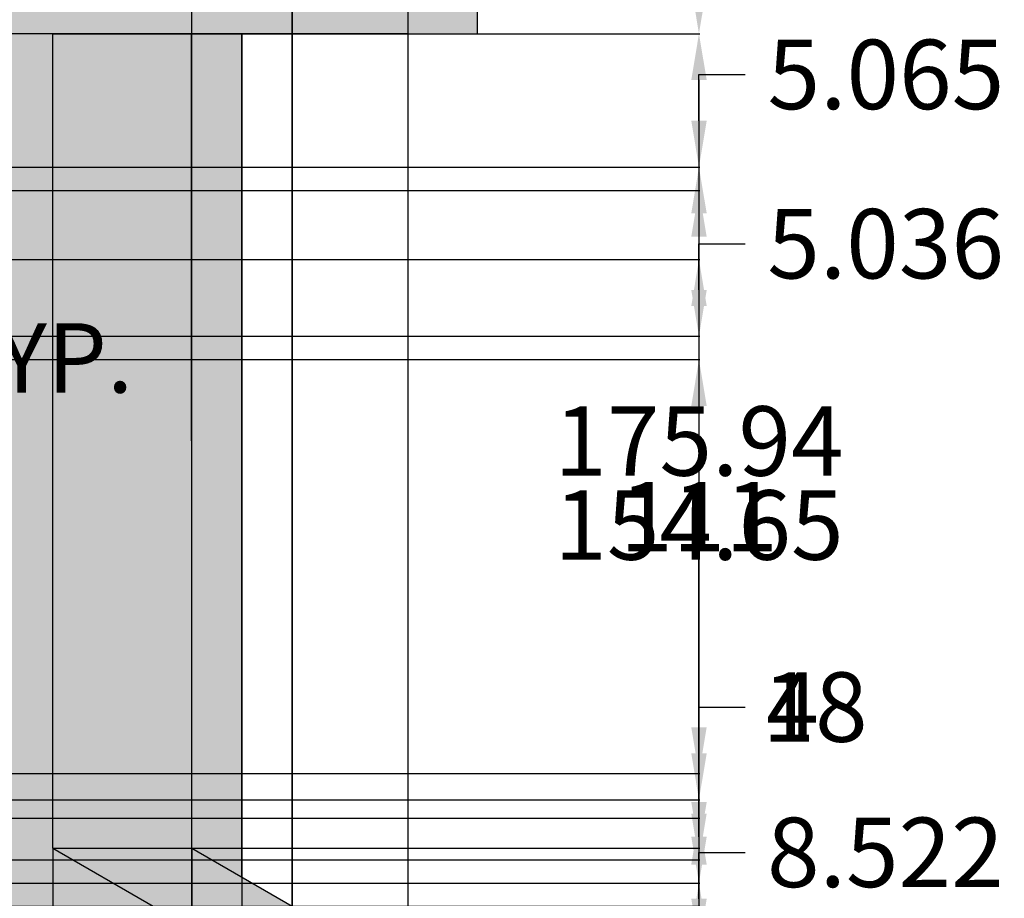
# Model space of a CAD drawing. Units: millimetres. Extents: x 131 to 845, y -20 to 1043.
# Tile 8 of 11: x 622 to 834, y 302 to 492. Entities that reach past the tile are written whole.
import ezdxf

# ---------------------------------------------------------------- set-up
doc = ezdxf.new("R2010")
doc.units = ezdxf.units.MM
doc.header["$MEASUREMENT"] = 0
for name, color, linetype, lineweight in [('A-ANNO-DIMS', 2, 'Continuous', 18), ('A-ELEV', 7, 'Continuous', 25), ('A-ELEV-PATT', 7, 'Continuous', 13), ('A-GLAZ-PATT', 143, 'Continuous', 13), ('A-WALL-PATT', 131, 'Continuous', 13)]:
    doc.layers.add(name, color=color, linetype=linetype, lineweight=lineweight)
doc.styles.get("Standard").update_dxf_attribs({"font": 'arial.ttf'})
doc.dimstyles.get("Standard").update_dxf_attribs({"dimtxt": 15, "dimasz": 10, "dimexe": 0.18, "dimexo": 0.0625, "dimgap": 5, "dimtad": 0, "dimtih": 1, "dimtoh": 1, "dimdec": 0, "dimzin": 0, "dimdsep": 46, "dimtxsty": 'Standard', "dimcen": 5, "dimadec": 0, "dimazin": 0, "dimtfac": 1, "dimtdec": 0, "dimtofl": 0, "dimtmove": 0, "dimatfit": 3, "dimfxl": 1, "dimtolj": 1, "dimtzin": 0, "dimarcsym": 0})

# ---------------------------------------------------------------- blocks, each defined once
blk = doc.blocks.new('*D12')
at = {"layer": 'A-ANNO-DIMS', "color": 0, "lineweight": -2, "transparency": 16777216}
for p, q in [((530.07, 423.18), (530.08, 418.34)), ((550.07, 423.21), (550.08, 418.36)), ((520.08, 418.5), (510.08, 418.49)), ((560.08, 418.56), (570.08, 418.57))]:
    blk.add_line(p, q, dxfattribs=at)
at = {"layer": 'A-ANNO-DIMS', "color": 0, "transparency": 16777216}
for points in [[(520.07, 420.17), (520.08, 416.83), (530.08, 418.52)], [(560.07, 420.22), (560.08, 416.89), (550.08, 418.54)]]:
    blk.add_solid(points, dxfattribs=at)
at = {"layer": 'Defpoints', "color": 0, "transparency": 16777216}
for p in [(530.07, 423.24), (550.07, 423.27), (550.08, 418.54)]:
    blk.add_point(p, dxfattribs=at)
at = {"layer": 'A-ANNO-DIMS', "color": 0, "transparency": 16777216, "insert": (611.71, 418.57), "char_height": 15, "attachment_point": 5}
blk.add_mtext('\\A1;20 TYP.', dxfattribs=at)
blk = doc.blocks.new('*D40')
at = {"layer": 'A-ANNO-DIMS', "color": 0, "lineweight": -2, "transparency": 16777216}
for p, q in [((720.6, 818.6), (768.56, 818.6)), ((768.38, 808.6), (768.38, 666.26)), ((768.38, 498.6), (768.38, 640.93)), ((720.6, 488.6), (768.56, 488.6))]:
    blk.add_line(p, q, dxfattribs=at)
at = {"layer": 'A-ANNO-DIMS', "color": 0, "transparency": 16777216}
for points in [[(766.72, 808.6), (770.05, 808.6), (768.38, 818.6)], [(766.72, 498.6), (770.05, 498.6), (768.38, 488.6)]]:
    blk.add_solid(points, dxfattribs=at)
at = {"layer": 'Defpoints', "color": 0, "transparency": 16777216}
for p in [(720.53, 818.6), (720.53, 488.6), (768.38, 488.6)]:
    blk.add_point(p, dxfattribs=at)
at = {"layer": 'A-ANNO-DIMS', "color": 0, "transparency": 16777216, "insert": (768.38, 653.6), "char_height": 15, "attachment_point": 5}
blk.add_mtext('\\A1;330', dxfattribs=at)
blk = doc.blocks.new('*D48')
at = {"layer": 'A-ANNO-DIMS', "color": 0, "lineweight": -2, "transparency": 16777216}
for p, q in [((680.53, 513.53), (680.53, -10.22)), ((705.53, 498.53), (705.53, -10.22)), ((670.53, -10.04), (660.53, -10.04)), ((715.53, -10.04), (725.53, -10.04))]:
    blk.add_line(p, q, dxfattribs=at)
at = {"layer": 'A-ANNO-DIMS', "color": 0, "transparency": 16777216}
for points in [[(670.53, -8.37), (670.53, -11.7), (680.53, -10.04)], [(715.53, -8.37), (715.53, -11.7), (705.53, -10.04)]]:
    blk.add_solid(points, dxfattribs=at)
at = {"layer": 'Defpoints', "color": 0, "transparency": 16777216}
for p in [(680.53, 513.6), (705.53, 498.6), (705.53, -10.04)]:
    blk.add_point(p, dxfattribs=at)
at = {"layer": 'A-ANNO-DIMS', "color": 0, "transparency": 16777216, "insert": (741.46, -10.04), "char_height": 15, "attachment_point": 5}
blk.add_mtext('\\A1;25', dxfattribs=at)
blk = doc.blocks.new('*D49')
at = {"layer": 'A-ANNO-DIMS', "color": 0, "lineweight": -2, "transparency": 16777216}
for p, q in [((768.38, 508.6), (768.38, 518.6)), ((768.38, 518.6), (778.38, 518.6)), ((705.6, 498.6), (768.56, 498.6)), ((720.6, 488.6), (768.56, 488.6)), ((768.38, 478.6), (768.38, 468.6))]:
    blk.add_line(p, q, dxfattribs=at)
at = {"layer": 'A-ANNO-DIMS', "color": 0, "transparency": 16777216}
for points in [[(766.72, 508.6), (770.05, 508.6), (768.38, 498.6)], [(766.72, 478.6), (770.05, 478.6), (768.38, 488.6)]]:
    blk.add_solid(points, dxfattribs=at)
at = {"layer": 'Defpoints', "color": 0, "transparency": 16777216}
for p in [(705.53, 498.6), (768.38, 498.6), (720.53, 488.6)]:
    blk.add_point(p, dxfattribs=at)
at = {"layer": 'A-ANNO-DIMS', "color": 0, "transparency": 16777216, "insert": (793.4, 518.6), "char_height": 15, "attachment_point": 5}
blk.add_mtext('\\A1;10', dxfattribs=at)
blk = doc.blocks.new('*D50')
at = {"layer": 'A-ANNO-DIMS', "color": 0, "lineweight": -2, "transparency": 16777216}
for p, q in [((720.6, 488.6), (768.56, 488.6)), ((768.38, 478.6), (768.38, 287.12)), ((768.38, 70.31), (768.38, 261.79)), ((216.3, 60.31), (768.56, 60.31))]:
    blk.add_line(p, q, dxfattribs=at)
at = {"layer": 'A-ANNO-DIMS', "color": 0, "transparency": 16777216}
for points in [[(766.72, 478.6), (770.05, 478.6), (768.38, 488.6)], [(766.72, 70.31), (770.05, 70.31), (768.38, 60.31)]]:
    blk.add_solid(points, dxfattribs=at)
at = {"layer": 'Defpoints', "color": 0, "transparency": 16777216}
for p in [(720.53, 488.6), (768.38, 488.6), (216.23, 60.31)]:
    blk.add_point(p, dxfattribs=at)
at = {"layer": 'A-ANNO-DIMS', "color": 0, "transparency": 16777216, "insert": (768.38, 274.45), "char_height": 15, "attachment_point": 5}
blk.add_mtext('\\A1;428.3', dxfattribs=at)
blk = doc.blocks.new('*D51')
at = {"layer": 'A-ANNO-DIMS', "color": 0, "lineweight": -2, "transparency": 16777216}
for p, q in [((658.81, 488.53), (658.81, -10.22)), ((628.88, 312.6), (628.88, -10.22)), ((618.88, -10.04), (608.88, -10.04)), ((668.81, -10.04), (678.81, -10.04))]:
    blk.add_line(p, q, dxfattribs=at)
at = {"layer": 'A-ANNO-DIMS', "color": 0, "transparency": 16777216}
for points in [[(618.88, -8.37), (618.88, -11.7), (628.88, -10.04)], [(668.81, -8.37), (668.81, -11.7), (658.81, -10.04)]]:
    blk.add_solid(points, dxfattribs=at)
at = {"layer": 'Defpoints', "color": 0, "transparency": 16777216}
for p in [(658.81, 488.6), (628.88, 312.66), (658.81, -10.04)]:
    blk.add_point(p, dxfattribs=at)
at = {"layer": 'A-ANNO-DIMS', "color": 0, "transparency": 16777216, "insert": (715.07, -10.04), "char_height": 15, "attachment_point": 5}
blk.add_mtext('\\A1;29.923', dxfattribs=at)
blk = doc.blocks.new('*D52')
at = {"layer": 'A-ANNO-DIMS', "color": 0, "lineweight": -2, "transparency": 16777216}
for p, q in [((669.71, 488.53), (669.71, -10.22)), ((658.88, 312.6), (658.88, -10.22)), ((648.88, -10.04), (638.88, -10.04)), ((679.71, -10.04), (689.71, -10.04))]:
    blk.add_line(p, q, dxfattribs=at)
at = {"layer": 'A-ANNO-DIMS', "color": 0, "transparency": 16777216}
for points in [[(648.88, -8.37), (648.88, -11.7), (658.88, -10.04)], [(679.71, -8.37), (679.71, -11.7), (669.71, -10.04)]]:
    blk.add_solid(points, dxfattribs=at)
at = {"layer": 'Defpoints', "color": 0, "transparency": 16777216}
for p in [(669.71, 488.6), (658.88, 312.66), (669.71, -10.04)]:
    blk.add_point(p, dxfattribs=at)
at = {"layer": 'A-ANNO-DIMS', "color": 0, "transparency": 16777216, "insert": (725.2, -10.04), "char_height": 15, "attachment_point": 5}
blk.add_mtext('\\A1;10.825', dxfattribs=at)
blk = doc.blocks.new('*D53')
at = {"layer": 'A-ANNO-DIMS', "color": 0, "lineweight": -2, "transparency": 16777216}
for p, q in [((628.95, 488.6), (768.56, 488.6)), ((768.38, 478.6), (768.38, 413.29)), ((768.38, 322.66), (768.38, 387.97)), ((628.95, 312.66), (768.56, 312.66))]:
    blk.add_line(p, q, dxfattribs=at)
at = {"layer": 'A-ANNO-DIMS', "color": 0, "transparency": 16777216}
for points in [[(766.72, 478.6), (770.05, 478.6), (768.38, 488.6)], [(766.72, 322.66), (770.05, 322.66), (768.38, 312.66)]]:
    blk.add_solid(points, dxfattribs=at)
at = {"layer": 'Defpoints', "color": 0, "transparency": 16777216}
for p in [(628.88, 488.6), (768.38, 488.6), (628.88, 312.66)]:
    blk.add_point(p, dxfattribs=at)
at = {"layer": 'A-ANNO-DIMS', "color": 0, "transparency": 16777216, "insert": (768.38, 400.63), "char_height": 15, "attachment_point": 5}
blk.add_mtext('\\A1;175.94', dxfattribs=at)
blk = doc.blocks.new('*D59')
at = {"layer": 'A-ANNO-DIMS', "color": 0, "lineweight": -2, "transparency": 16777216}
for p, q in [((615.11, 459.8), (768.56, 459.8)), ((768.38, 449.8), (768.38, 395.14)), ((768.38, 315.16), (768.38, 369.82)), ((617.11, 305.16), (768.56, 305.16))]:
    blk.add_line(p, q, dxfattribs=at)
at = {"layer": 'A-ANNO-DIMS', "color": 0, "transparency": 16777216}
for points in [[(766.72, 449.8), (770.05, 449.8), (768.38, 459.8)], [(766.72, 315.16), (770.05, 315.16), (768.38, 305.16)]]:
    blk.add_solid(points, dxfattribs=at)
at = {"layer": 'Defpoints', "color": 0, "transparency": 16777216}
for p in [(615.05, 459.8), (617.05, 305.16), (768.38, 305.16)]:
    blk.add_point(p, dxfattribs=at)
at = {"layer": 'A-ANNO-DIMS', "color": 0, "transparency": 16777216, "insert": (768.38, 382.48), "char_height": 15, "attachment_point": 5}
blk.add_mtext('\\A1;154.65', dxfattribs=at)
blk = doc.blocks.new('*D60')
at = {"layer": 'A-ANNO-DIMS', "color": 0, "lineweight": -2, "transparency": 16777216}
for p, q in [((768.38, 333.16), (768.38, 343.16)), ((768.38, 343.16), (778.38, 343.16)), ((617.11, 323.16), (768.56, 323.16)), ((617.11, 305.16), (768.56, 305.16)), ((768.38, 295.16), (768.38, 285.16))]:
    blk.add_line(p, q, dxfattribs=at)
at = {"layer": 'A-ANNO-DIMS', "color": 0, "transparency": 16777216}
for points in [[(766.72, 333.16), (770.05, 333.16), (768.38, 323.16)], [(766.72, 295.16), (770.05, 295.16), (768.38, 305.16)]]:
    blk.add_solid(points, dxfattribs=at)
at = {"layer": 'Defpoints', "color": 0, "transparency": 16777216}
for p in [(617.05, 323.16), (768.38, 323.16), (617.05, 305.16)]:
    blk.add_point(p, dxfattribs=at)
at = {"layer": 'A-ANNO-DIMS', "color": 0, "transparency": 16777216, "insert": (793.44, 343.16), "char_height": 15, "attachment_point": 5}
blk.add_mtext('\\A1;18', dxfattribs=at)
blk = doc.blocks.new('*D61')
at = {"layer": 'A-ANNO-DIMS', "color": 0, "lineweight": -2, "transparency": 16777216}
for p, q in [((768.38, 333.16), (768.38, 343.16)), ((768.38, 343.16), (778.38, 343.16)), ((617.11, 323.16), (768.56, 323.16)), ((617.11, 319.16), (768.56, 319.16)), ((768.38, 309.16), (768.38, 299.16))]:
    blk.add_line(p, q, dxfattribs=at)
at = {"layer": 'A-ANNO-DIMS', "color": 0, "transparency": 16777216}
for points in [[(766.72, 333.16), (770.05, 333.16), (768.38, 323.16)], [(766.72, 309.16), (770.05, 309.16), (768.38, 319.16)]]:
    blk.add_solid(points, dxfattribs=at)
at = {"layer": 'Defpoints', "color": 0, "transparency": 16777216}
for p in [(617.05, 323.16), (768.38, 323.16), (617.05, 319.16)]:
    blk.add_point(p, dxfattribs=at)
at = {"layer": 'A-ANNO-DIMS', "color": 0, "transparency": 16777216, "insert": (788.57, 343.16), "char_height": 15, "attachment_point": 5}
blk.add_mtext('\\A1;4', dxfattribs=at)
blk = doc.blocks.new('*D63')
at = {"layer": 'A-ANNO-DIMS', "color": 0, "lineweight": -2, "transparency": 16777216}
for p, q in [((768.38, 469.8), (768.38, 479.8)), ((768.38, 479.8), (778.38, 479.8)), ((525.11, 459.8), (768.56, 459.8)), ((530.09, 454.74), (768.56, 454.74)), ((768.38, 444.74), (768.38, 434.74))]:
    blk.add_line(p, q, dxfattribs=at)
at = {"layer": 'A-ANNO-DIMS', "color": 0, "transparency": 16777216}
for points in [[(766.72, 469.8), (770.05, 469.8), (768.38, 459.8)], [(766.72, 444.74), (770.05, 444.74), (768.38, 454.74)]]:
    blk.add_solid(points, dxfattribs=at)
at = {"layer": 'Defpoints', "color": 0, "transparency": 16777216}
for p in [(525.05, 459.8), (768.38, 459.8), (530.02, 454.74)]:
    blk.add_point(p, dxfattribs=at)
at = {"layer": 'A-ANNO-DIMS', "color": 0, "transparency": 16777216, "insert": (808.75, 479.8), "char_height": 15, "attachment_point": 5}
blk.add_mtext('\\A1;5.065', dxfattribs=at)
blk = doc.blocks.new('*D64')
at = {"layer": 'A-ANNO-DIMS', "color": 0, "lineweight": -2, "transparency": 16777216}
for p, q in [((768.38, 433.24), (768.38, 443.24)), ((768.38, 443.24), (778.38, 443.24)), ((530.13, 423.24), (768.56, 423.24)), ((530.11, 418.2), (768.56, 418.2)), ((768.38, 408.2), (768.38, 398.2))]:
    blk.add_line(p, q, dxfattribs=at)
at = {"layer": 'A-ANNO-DIMS', "color": 0, "transparency": 16777216}
for points in [[(766.72, 433.24), (770.05, 433.24), (768.38, 423.24)], [(766.72, 408.2), (770.05, 408.2), (768.38, 418.2)]]:
    blk.add_solid(points, dxfattribs=at)
at = {"layer": 'Defpoints', "color": 0, "transparency": 16777216}
for p in [(530.07, 423.24), (768.38, 423.24), (530.05, 418.2)]:
    blk.add_point(p, dxfattribs=at)
at = {"layer": 'A-ANNO-DIMS', "color": 0, "transparency": 16777216, "insert": (808.69, 443.24), "char_height": 15, "attachment_point": 5}
blk.add_mtext('\\A1;5.036', dxfattribs=at)
blk = doc.blocks.new('*D66')
at = {"layer": 'A-ANNO-DIMS', "color": 0, "lineweight": -2, "transparency": 16777216}
for p, q in [((563.11, 439.8), (768.56, 439.8)), ((768.38, 429.8), (768.38, 396.84)), ((768.38, 338.8), (768.38, 371.77)), ((563.11, 328.8), (768.56, 328.8))]:
    blk.add_line(p, q, dxfattribs=at)
at = {"layer": 'A-ANNO-DIMS', "color": 0, "transparency": 16777216}
for points in [[(766.72, 429.8), (770.05, 429.8), (768.38, 439.8)], [(766.72, 338.8), (770.05, 338.8), (768.38, 328.8)]]:
    blk.add_solid(points, dxfattribs=at)
at = {"layer": 'Defpoints', "color": 0, "transparency": 16777216}
for p in [(563.05, 439.8), (768.38, 439.8), (563.05, 328.8)]:
    blk.add_point(p, dxfattribs=at)
at = {"layer": 'A-ANNO-DIMS', "color": 0, "transparency": 16777216, "insert": (768.38, 384.3), "char_height": 15, "attachment_point": 5}
blk.add_mtext('\\A1;111', dxfattribs=at)
blk = doc.blocks.new('*D69')
at = {"layer": 'A-ANNO-DIMS', "color": 0, "lineweight": -2, "transparency": 16777216}
for p, q in [((570.05, 303.56), (570.05, -10.22)), ((572.05, 303.56), (572.05, -10.22)), ((560.05, -10.04), (550.05, -10.04)), ((582.05, -10.04), (592.05, -10.04))]:
    blk.add_line(p, q, dxfattribs=at)
at = {"layer": 'A-ANNO-DIMS', "color": 0, "transparency": 16777216}
for points in [[(560.05, -8.37), (560.05, -11.7), (570.05, -10.04)], [(582.05, -8.37), (582.05, -11.7), (572.05, -10.04)]]:
    blk.add_solid(points, dxfattribs=at)
at = {"layer": 'Defpoints', "color": 0, "transparency": 16777216}
for p in [(570.05, 303.62), (572.05, 303.62), (572.05, -10.04)]:
    blk.add_point(p, dxfattribs=at)
at = {"layer": 'A-ANNO-DIMS', "color": 0, "transparency": 16777216, "insert": (616.63, -10.04), "char_height": 15, "attachment_point": 5}
blk.add_mtext('\\A1;2.00', dxfattribs=at)
blk = doc.blocks.new('*D76')
at = {"layer": 'A-ANNO-DIMS', "color": 0, "lineweight": -2, "transparency": 16777216}
for p, q in [((768.38, 320.16), (768.38, 330.16)), ((472.3, 310.16), (768.56, 310.16)), ((489.62, 300.16), (768.56, 300.16)), ((768.38, 290.16), (768.38, 280.16)), ((768.38, 280.16), (758.38, 280.16))]:
    blk.add_line(p, q, dxfattribs=at)
at = {"layer": 'A-ANNO-DIMS', "color": 0, "transparency": 16777216}
for points in [[(766.72, 320.16), (770.05, 320.16), (768.38, 310.16)], [(766.72, 290.16), (770.05, 290.16), (768.38, 300.16)]]:
    blk.add_solid(points, dxfattribs=at)
at = {"layer": 'Defpoints', "color": 0, "transparency": 16777216}
for p in [(472.24, 310.16), (489.56, 300.16), (768.38, 300.16)]:
    blk.add_point(p, dxfattribs=at)
at = {"layer": 'A-ANNO-DIMS', "color": 0, "transparency": 16777216, "insert": (743.37, 280.16), "char_height": 15, "attachment_point": 5}
blk.add_mtext('\\A1;10', dxfattribs=at)
blk = doc.blocks.new('*D77')
at = {"layer": 'A-ANNO-DIMS', "color": 0, "lineweight": -2, "transparency": 16777216}
for p, q in [((648.88, 1033.52), (638.88, 1033.52)), ((658.88, 312.72), (658.88, 1033.7)), ((680.53, 300.22), (680.53, 1033.7)), ((690.53, 1033.52), (700.53, 1033.52))]:
    blk.add_line(p, q, dxfattribs=at)
at = {"layer": 'A-ANNO-DIMS', "color": 0, "transparency": 16777216}
for points in [[(648.88, 1035.18), (648.88, 1031.85), (658.88, 1033.52)], [(690.53, 1035.18), (690.53, 1031.85), (680.53, 1033.52)]]:
    blk.add_solid(points, dxfattribs=at)
at = {"layer": 'Defpoints', "color": 0, "transparency": 16777216}
for p in [(680.53, 1033.52), (658.88, 312.66), (680.53, 300.16)]:
    blk.add_point(p, dxfattribs=at)
at = {"layer": 'A-ANNO-DIMS', "color": 0, "transparency": 16777216, "insert": (731.03, 1033.52), "char_height": 15, "attachment_point": 5}
blk.add_mtext('\\A1;21.65', dxfattribs=at)
blk = doc.blocks.new('*D78')
at = {"layer": 'A-ANNO-DIMS', "color": 0, "lineweight": -2, "transparency": 16777216}
for p, q in [((768.38, 322.66), (768.38, 332.66)), ((658.95, 312.66), (768.56, 312.66)), ((680.6, 300.16), (768.56, 300.16)), ((768.38, 290.16), (768.38, 280.16)), ((768.38, 280.16), (758.38, 280.16))]:
    blk.add_line(p, q, dxfattribs=at)
at = {"layer": 'A-ANNO-DIMS', "color": 0, "transparency": 16777216}
for points in [[(766.72, 322.66), (770.05, 322.66), (768.38, 312.66)], [(766.72, 290.16), (770.05, 290.16), (768.38, 300.16)]]:
    blk.add_solid(points, dxfattribs=at)
at = {"layer": 'Defpoints', "color": 0, "transparency": 16777216}
for p in [(658.88, 312.66), (680.53, 300.16), (768.38, 300.16)]:
    blk.add_point(p, dxfattribs=at)
at = {"layer": 'A-ANNO-DIMS', "color": 0, "transparency": 16777216, "insert": (734.55, 280.16), "char_height": 15, "attachment_point": 5}
blk.add_mtext('\\A1;12.5', dxfattribs=at)
blk = doc.blocks.new('*D85')
at = {"layer": 'A-ANNO-DIMS', "color": 0, "lineweight": -2, "transparency": 16777216}
for p, q in [((768.38, 301.78), (768.38, 311.78)), ((768.38, 311.78), (778.38, 311.78)), ((639.93, 291.78), (768.56, 291.78)), ((602.06, 283.26), (768.56, 283.26)), ((768.38, 273.26), (768.38, 263.26))]:
    blk.add_line(p, q, dxfattribs=at)
at = {"layer": 'A-ANNO-DIMS', "color": 0, "transparency": 16777216}
for points in [[(766.72, 301.78), (770.05, 301.78), (768.38, 291.78)], [(766.72, 273.26), (770.05, 273.26), (768.38, 283.26)]]:
    blk.add_solid(points, dxfattribs=at)
at = {"layer": 'Defpoints', "color": 0, "transparency": 16777216}
for p in [(639.87, 291.78), (768.38, 291.78), (601.99, 283.26)]:
    blk.add_point(p, dxfattribs=at)
at = {"layer": 'A-ANNO-DIMS', "color": 0, "transparency": 16777216, "insert": (808.63, 311.78), "char_height": 15, "attachment_point": 5}
blk.add_mtext('\\A1;8.522', dxfattribs=at)

msp = doc.modelspace()

# ---------------------------------------------------------------- hatches: boundary and pattern name
at = {"layer": 'A-ELEV-PATT', "transparency": 33554681}
h = msp.add_hatch(color=256, dxfattribs=at)
h.set_gradient(color1=(255, 255, 255), color2=(199, 200, 202), name='INVSPHERICAL')
h.paths.add_polyline_path([(459.5586, 310.1596), (472.2381, 310.1596), (489.5586, 300.1596), (650.5349, 300.1596), (628.8842, 312.6596), (628.8842, 488.5953), (459.5586, 488.5953)])
h.paths.add_polyline_path([(525.0467, 459.8046), (615.0467, 459.8046), (615.0467, 323.1596), (617.0467, 323.1596), (617.0467, 319.1596), (615.0467, 319.1596), (615.0467, 309.1596), (617.0467, 309.1596), (617.0467, 305.1596), (572.0467, 305.1596), (572.0453, 303.6234), (570.0467, 303.6234), (570.0467, 305.1596), (525.0467, 305.1596), (523.0467, 305.1596), (523.0467, 309.1596), (525.0467, 309.1596), (525.0467, 319.1596), (523.0467, 319.1596), (523.0467, 323.1596), (525.0467, 323.1596)], flags=16)
h.paths.add_polyline_path([(530.0467, 454.8046), (550.0467, 454.8046), (550.0467, 423.2044), (530.0467, 423.2044)], flags=0)
h.paths.add_polyline_path([(530.0467, 418.2044), (550.0467, 418.2044), (550.0467, 386.7044), (530.0467, 386.7044)], flags=0)
h.paths.add_polyline_path([(560.0467, 439.8046), (563.0467, 439.8046), (563.0467, 328.8046), (560.0467, 328.8046)], flags=0)
h.paths.add_polyline_path([(530.0467, 381.7044), (550.0467, 381.7044), (550.0467, 350.2044), (530.0467, 350.2044)], flags=0)
h.paths.add_polyline_path([(554.0467, 319.1596), (554.0467, 315.1596), (540.0467, 315.1596), (540.0467, 313.7044), (530.0467, 313.7044), (530.0467, 319.1596)], flags=0)
h.paths.add_polyline_path([(556.0467, 319.1596), (561.0467, 319.1596), (561.0467, 315.1596), (556.0467, 315.1596)], flags=0)
h.paths.add_polyline_path([(563.0467, 319.1596), (568.0467, 319.1596), (568.0467, 315.1596), (563.0467, 315.1596)], flags=0)
h.paths.add_polyline_path([(556.0467, 313.1596), (561.0467, 313.1596), (561.0467, 309.1596), (556.0467, 309.1596)], flags=0)
h.paths.add_polyline_path([(563.0467, 313.1596), (568.0467, 313.1596), (568.0467, 309.1596), (563.0467, 309.1596)], flags=0)
h.paths.add_polyline_path([(574.0467, 319.1596), (579.0467, 319.1596), (579.0467, 315.1596), (574.1854, 315.1596), (574.1854, 313.1596), (579.0467, 313.1596), (579.0467, 309.1596), (574.0467, 309.1596), (574.0467, 313.1596), (574.1854, 315.1596), (574.0467, 315.1596)], flags=0)
h.paths.add_polyline_path([(581.0467, 319.1596), (586.0467, 319.1596), (586.0467, 315.1596), (581.0467, 315.1596)], flags=0)
h.paths.add_polyline_path([(581.0467, 313.1596), (586.0467, 313.1596), (586.0467, 309.1596), (581.0467, 309.1596)], flags=0)
h = msp.add_hatch(color=256, dxfattribs=at)
h.set_gradient(color1=(199, 200, 202), color2=(147, 149, 152), name='INVSPHERICAL')
h.paths.add_polyline_path([(669.7096, 488.5953), (658.8074, 488.5953), (658.8842, 312.6596), (669.7096, 306.4096)])
h = msp.add_hatch(color=256, dxfattribs=at)
h.set_gradient(color1=(79, 2, 22), color2=(153, 133, 76), name='SPHERICAL')
h.paths.add_polyline_path([(459.5586, 310.1596), (459.5586, 300.1596), (489.5586, 300.1596), (472.2381, 310.1596)])
h.paths.add_polyline_path([(658.8842, 312.6596), (628.8842, 312.6596), (650.5349, 300.1596), (680.5349, 300.1596)])
at = {"layer": 'A-GLAZ-PATT'}
h = msp.add_hatch(color=256, dxfattribs=at)
h.dxf.hatch_style = 1
h.paths.add_polyline_path([(658.8074, 488.5953), (628.8842, 488.5953), (628.8842, 312.6596), (658.8842, 312.6596)])
h.paths.add_polyline_path([(650.5349, 97.8131), (459.5586, 97.8131), (459.5586, 82.8131), (658.5215, 82.8131)])
h.paths.add_polyline_path([(658.5215, 67.8131), (459.5586, 67.8131), (459.5586, 52.8131), (663.9762, 52.8131)])
at = {"layer": 'A-WALL-PATT'}
h = msp.add_hatch(color=256, dxfattribs=at)
h.dxf.hatch_style = 1
h.paths.add_polyline_path([(449.5586, 833.5953), (451.6297, 835.6663), (451.6297, 885.6663), (466.6297, 885.6663), (466.6297, 891.3345), (330.6595, 891.3345), (330.6595, 856.8345), (292.1595, 856.8345), (292.1595, 798.4332), (336.1595, 798.4332), (336.1595, 178.4332), (246.1595, 178.4332), (246.1595, 798.4332), (290.1595, 798.4332), (290.1595, 856.8345), (259.6595, 856.8345), (255.6595, 860.8345), (255.6595, 927.8345), (290.1595, 927.8345), (290.1595, 960.6663), (216.2327, 960.6663), (216.2327, 60.3131), (459.5586, 60.3131), (459.5586, 97.8131), (459.5586, 252.07), (459.5586, 283.5561), (369.5586, 283.5561), (369.5586, 763.5561), (439.5586, 763.5561), (439.5586, 778.6714), (439.5586, 793.5953), (439.5586, 796.5953), (441.5586, 798.5953), (444.5586, 798.5953), (444.5586, 813.5953), (444.5586, 816.5953), (446.5586, 818.5953), (449.5586, 818.5953)])
h.paths.add_polyline_path([(466.6297, 960.6663), (292.1595, 960.6663), (292.1595, 927.8345), (326.6595, 927.8345), (330.6595, 923.8345), (330.6595, 893.3345), (466.6297, 893.3345)], flags=17)
h.paths.add_polyline_path([(720.5349, 813.5953), (720.5349, 818.5953), (710.5349, 818.5953), (449.5586, 818.5953), (446.5586, 818.5953), (444.5586, 816.5953), (444.5586, 813.5953), (444.5586, 798.5953), (705.5349, 798.5953), (705.5349, 513.5953), (705.5349, 498.5953), (680.5349, 498.5953), (680.5349, 488.5953), (705.5349, 488.5953), (720.5349, 488.5953), (720.5349, 513.5953)])
h.paths.add_polyline_path([(680.5349, 498.5953), (412.6606, 498.5953), (412.6606, 488.5953), (680.5349, 488.5953)])

# ---------------------------------------------------------------- linework, layer by layer
at = {"layer": 'A-ELEV'}
for p, q in [((720.5349, 488.5953), (720.5349, 513.5953)), ((680.5349, 498.5953), (680.5349, 488.5953)), ((705.5349, 488.5953), (412.6606, 488.5953)), ((628.8842, 312.6596), (628.8842, 488.5953)), ((658.8842, 312.6596), (658.8074, 488.5953)), ((669.7096, 306.4096), (669.7096, 488.5953)), ((705.5349, 488.5953), (720.5349, 488.5953)), ((628.8842, 312.6596), (658.8842, 312.6596)), ((628.8842, 312.6596), (650.5349, 300.1596)), ((658.8842, 312.6596), (680.5349, 300.1596))]:
    msp.add_line(p, q, dxfattribs=at)

# ---------------------------------------------------------------- dimensions: what is measured, and where the dimension line sits
at = {"layer": 'A-ANNO-DIMS'}
for base, p1, p2, override, picture, middle in [((680.5349, 1033.5163), (658.8842, 312.6596), (680.5349, 300.1596), {"dimdec": 2, "dimlfac": 1, "dimrnd": 0, "dimzin": 0, "dimdsep": 46, "dimlunit": 2}, '*D77', (731.0277, 1033.5163)), ((705.5349, -10.0369), (680.5349, 513.5953), (705.5349, 498.5953), {"dimdec": 0, "dimlfac": 1, "dimrnd": 0, "dimzin": 0, "dimdsep": 46, "dimlunit": 2}, '*D48', (741.4626, -10.0369)), ((658.8074, -10.0369), (628.8842, 312.6596), (658.8074, 488.5953), {"dimdec": 3, "dimlfac": 1, "dimrnd": 0, "dimzin": 0, "dimdsep": 46, "dimlunit": 2}, '*D51', (715.0711, -10.0369)), ((669.7096, -10.0369), (658.8842, 312.6596), (669.7096, 488.5953), {"dimdec": 3, "dimlfac": 1, "dimrnd": 0, "dimzin": 0, "dimdsep": 46, "dimlunit": 2}, '*D52', (725.1956, -10.0369)), ((572.0453, -10.0369), (570.0467, 303.6234), (572.0453, 303.6234), {"dimdec": 2, "dimlfac": 1, "dimrnd": 0, "dimzin": 0, "dimdsep": 46, "dimlunit": 2}, '*D69', (616.6292, -10.0369))]:
    dim = msp.add_linear_dim(base=base, p1=p1, p2=p2, dimstyle='Standard', override=override, dxfattribs=at)
    dim.commit()
    dim.dimension.update_dxf_attribs({"geometry": picture, "text_midpoint": middle})
for base, p1, p2, override, picture, middle in [((768.3849, 488.5953), (720.5349, 818.5953), (720.5349, 488.5953), {"dimdec": 0, "dimlfac": 1, "dimrnd": 0, "dimzin": 0, "dimdsep": 46, "dimlunit": 2}, '*D40', (768.3849, 653.5953)), ((768.3849, 498.5953), (720.5349, 488.5953), (705.5349, 498.5953), {"dimdec": 0, "dimlfac": 1, "dimrnd": 0, "dimzin": 0, "dimdsep": 46, "dimlunit": 2}, '*D49', (793.3968, 518.5953)), ((768.38488, 459.80465), (530.0241, 454.74011), (525.04673, 459.80464), {"dimdec": 3, "dimlfac": 1, "dimrnd": 0, "dimzin": 0, "dimdsep": 46, "dimlunit": 2}, '*D63', (808.74982, 479.80464)), ((768.3849, 488.5953), (216.2327, 60.3131), (720.5349, 488.5953), {"dimdec": 1, "dimlfac": 1, "dimrnd": 0, "dimzin": 0, "dimdsep": 46, "dimlunit": 2}, '*D50', (768.3849, 274.4542)), ((768.3849, 488.5953), (628.8842, 312.6596), (628.8842, 488.5953), {"dimdec": 2, "dimlfac": 1, "dimrnd": 0, "dimzin": 0, "dimdsep": 46, "dimlunit": 2}, '*D53', (768.3849, 400.6274)), ((768.38488, 305.1596), (615.04673, 459.80464), (617.04673, 305.1596), {"dimdec": 2, "dimlfac": 1, "dimrnd": 0, "dimzin": 0, "dimdsep": 46, "dimlunit": 2}, '*D59', (768.38488, 382.48212)), ((768.3849, 423.2401), (530.0467, 418.2044), (530.0694, 423.2401), {"dimdec": 3, "dimlfac": 1, "dimrnd": 0, "dimzin": 0, "dimdsep": 46, "dimlunit": 2}, '*D64', (808.6884, 443.2401)), ((768.3849, 439.8046), (563.0467, 328.8046), (563.0467, 439.8046), {"dimdec": 0, "dimlfac": 1, "dimrnd": 0, "dimzin": 0, "dimdsep": 46, "dimlunit": 2}, '*D66', (768.3849, 384.3046)), ((768.3849, 323.1596), (617.0467, 305.1596), (617.0467, 323.1596), {"dimdec": 0, "dimlfac": 1, "dimrnd": 0, "dimzin": 0, "dimdsep": 46, "dimlunit": 2}, '*D60', (793.4377, 343.1596)), ((768.3849, 323.1596), (617.0467, 319.1596), (617.0467, 323.1596), {"dimdec": 0, "dimlfac": 1, "dimrnd": 0, "dimzin": 0, "dimdsep": 46, "dimlunit": 2}, '*D61', (788.5725, 343.1596)), ((768.3849, 300.1596), (658.8842, 312.6596), (680.5349, 300.1596), {"dimdec": 1, "dimlfac": 1, "dimrnd": 0, "dimzin": 0, "dimdsep": 46, "dimlunit": 2}, '*D78', (734.553, 280.1596)), ((768.3849, 300.1596), (472.2381, 310.1596), (489.5586, 300.1596), {"dimdec": 0, "dimlfac": 1, "dimrnd": 0, "dimzin": 0, "dimdsep": 46, "dimlunit": 2}, '*D76', (743.3729, 280.1596)), ((768.3849, 291.7824), (601.9946, 283.2603), (639.8713, 291.7824), {"dimdec": 3, "dimlfac": 1, "dimrnd": 0, "dimzin": 0, "dimdsep": 46, "dimlunit": 2}, '*D85', (808.627, 311.7824))]:
    dim = msp.add_linear_dim(base=base, p1=p1, p2=p2, angle=90, dimstyle='Standard', override=override, dxfattribs=at)
    dim.commit()
    dim.dimension.update_dxf_attribs({"geometry": picture, "text_midpoint": middle})
dim = msp.add_linear_dim(base=(550.0762, 418.5439), p1=(530.0694, 423.2401), p2=(550.0694, 423.2689), angle=0.082356, text='<> TYP.', dimstyle='Standard', override={"dimdec": 0, "dimrnd": 0, "dimzin": 0, "dimlunit": 2}, dxfattribs=at)
dim.commit()
dim.dimension.update_dxf_attribs({"geometry": '*D12', "text_midpoint": (611.7115, 418.5726)})

doc.saveas('drawing.dxf')
